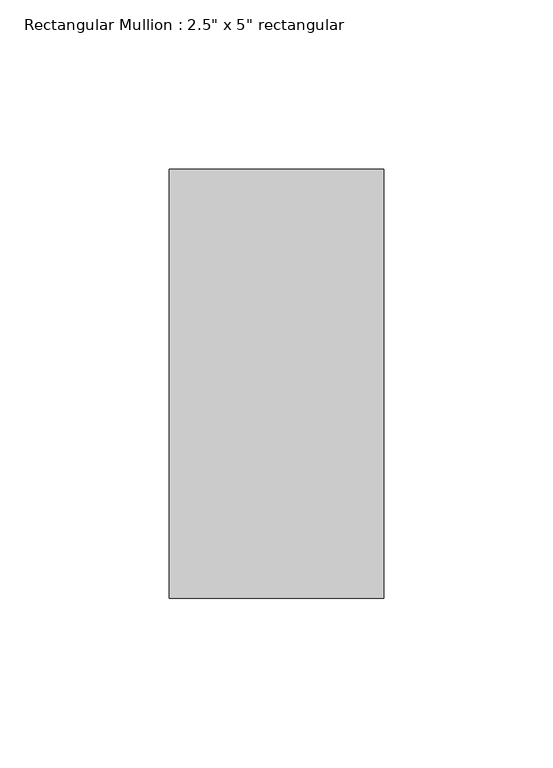
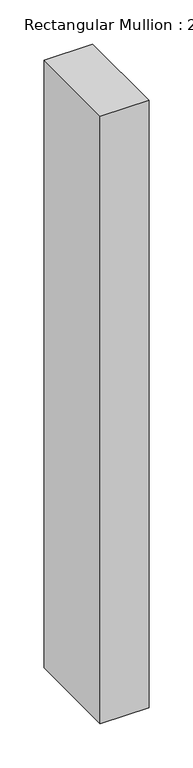
"""IFC4 building model written with IfcOpenShell, lengths in millimetres: member geometry."""

from ifc_helpers import new_model, si_unit, frame, origin, place, context, project, spatial, polyline, outline, extrude, source, transform, mapped, element, save


def member_1bc815af(model_context):
    return source(origin(), model_context, "Body", "SweptSolid", [
        extrude(outline(polyline([(31.75, 63.5), (31.75, -63.5), (-31.75, -63.5), (-31.75, 63.5), (31.75, 63.5)])), frame((0.0, 0.0, -837.8574877), z_axis=(0.0, 0.0, 1.0), x_axis=(1.0, 0.0, 0.0)), (0.0, 0.0, 1.0), 837.8574877),
    ])


if __name__ == "__main__":
    model = new_model("IFC4")
    model_context = context("Model", 3, world=origin())
    ifc_project = project(units=[si_unit("LENGTHUNIT", "METRE", prefix="MILLI")], contexts=[model_context])
    site = spatial("IfcSite", under=ifc_project)
    building = spatial("IfcBuilding", under=site)
    placement = place(None, origin())
    member_shape = member_1bc815af(model_context)
    element("IfcMember", 1, ObjectType="Rectangular Mullion : 2.5\" x 5\" rectangular", at=placement, inside=building, context=model_context, shape_type="MappedRepresentation", body=[
        mapped(member_shape, transform((0.0, 0.0, 0.0), x_axis=(1.0, 0.0, 0.0), y_axis=(0.0, 1.0, 0.0), z_axis=(0.0, 0.0, 1.0))),
    ])
    save(model, "model.ifc")

# Revit data of these elements
# Type "Rectangular Mullion : 2.5\" x 5\" rectangular"
#   built-in parameter 1007304 = 0.416667 (stored number, unit not read)
#   built-in parameter 1007301 = 0.104167 (stored number, unit not read)
#   built-in parameter 1007300 = 0.104167 (stored number, unit not read)
# Element 1 (IfcMember, "Rectangular Mullion : 2.5\" x 5\" rectangular")
#   Materials on its faces: "Aluminum"
# Materials
#   "Aluminum": class "Metal", colour RGB 247 247 247, transparency 0, Description = "Aluminum 6061", Cost = 0
